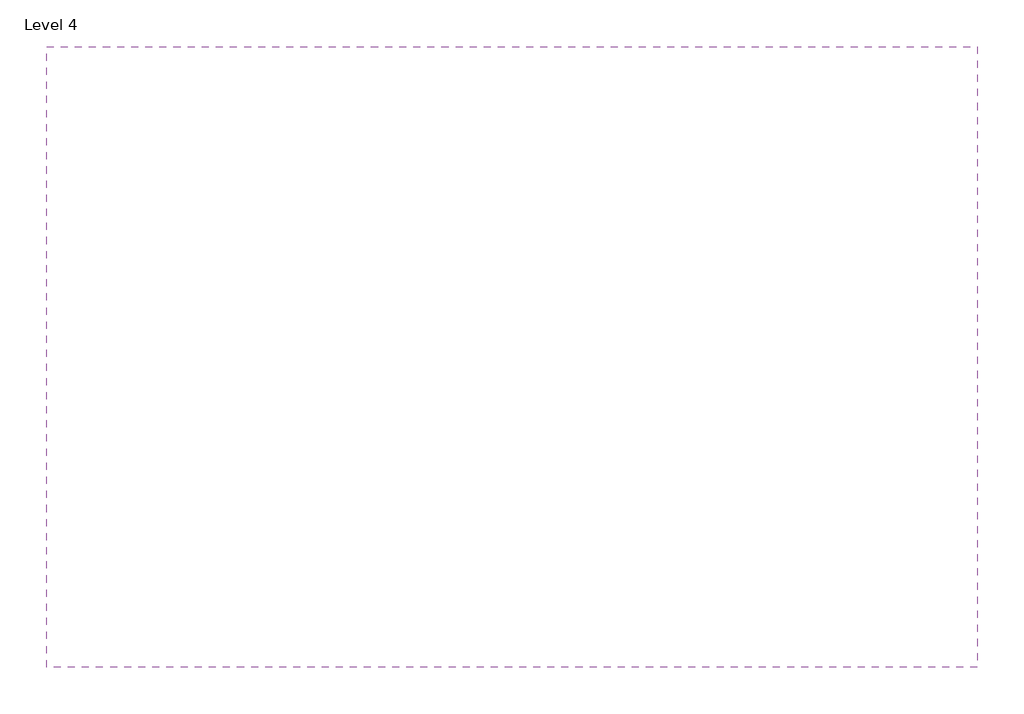
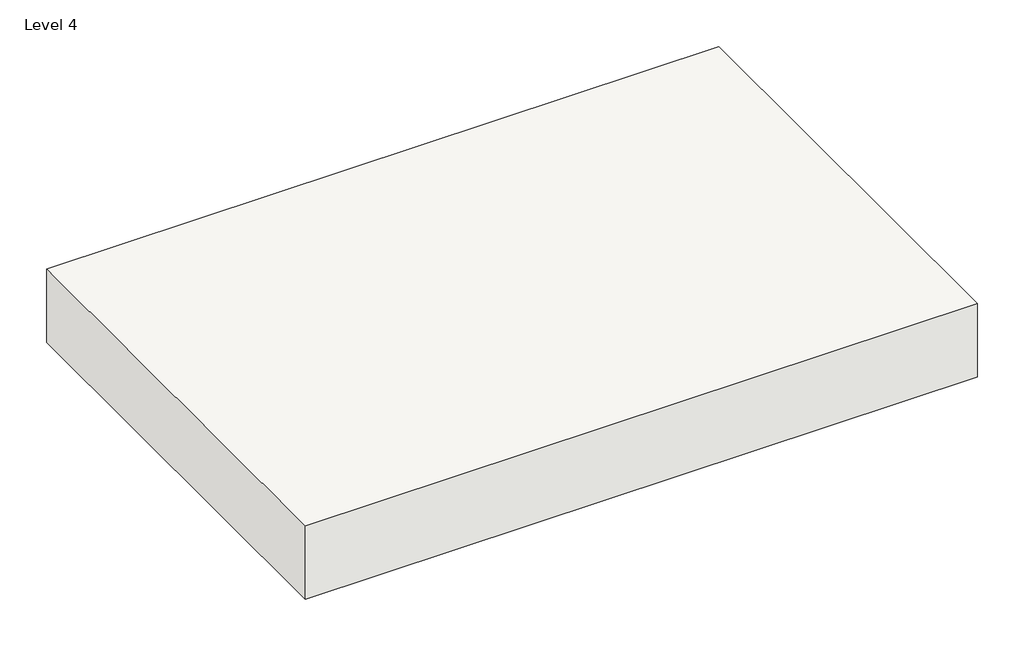
# One storey: 1 slab.
"""IFC4 building model written with IfcOpenShell, lengths in millimetres."""

from ifc_helpers import new_model, si_unit, frame, origin, place, context, project, spatial, polyline, outline, extrude, element, save

model = new_model("IFC4")

# Units and contexts
model_context = context("Model", 3, world=origin())
ifc_project = project(units=[si_unit("LENGTHUNIT", "METRE", prefix="MILLI")], contexts=[model_context])

# Site, building, storey
site = spatial("IfcSite", under=ifc_project)
building = spatial("IfcBuilding", under=site)
storey = spatial("IfcBuildingStorey", under=building, Name="Level 4", Elevation=3962.4)

# Slab
placement = place(None, origin())
element("IfcSlab", 1, ObjectType="slab 6\"", at=placement, inside=storey, context=model_context, shape_type="SweptSolid", body=[
    extrude(outline(polyline([(-622.2766939, 3731.7902438), (-622.2766939, 1979.1902438), (-3251.1766939, 1979.1902438), (-3251.1766939, 3731.7902438), (-622.2766939, 3731.7902438)])), frame((0.0, 0.0, 5181.6), z_axis=(0.0, 0.0, 1.0), x_axis=(1.0, 0.0, 0.0)), (0.0, 0.0, 1.0), 304.8),
])

save(model, "model.ifc")

# Revit data of these elements
# Type "slab 6\""
#   Assembly Code = "B1010"
#   Function = 0
#   Layers, outside or top first: 1' - 0" no material (function 1)
# Element 1 (IfcSlab, "slab 6\"")
#   Height Offset From Level = 5' - 0"
#   Phase Created = New Construction
#   Materials on its faces: "Default Floor"
# Materials
#   "Default Floor": colour RGB 128 128 128, transparency 0, Cost = 0
